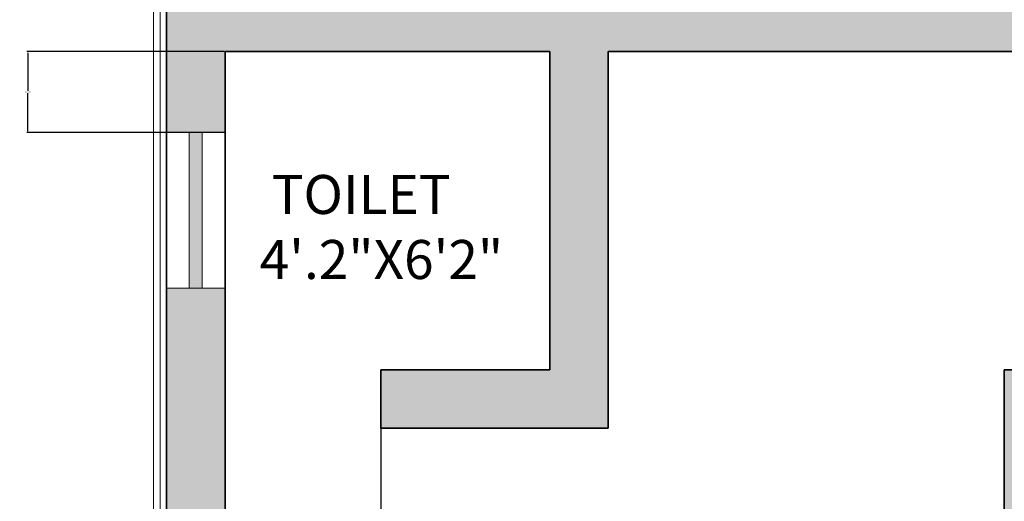
# Model space of a CAD drawing. Units: inches. Extents: x 311 to 815, y -527 to 136.
# Tile 6 of 21: x 388 to 539, y -368 to -294. Entities that reach past the tile are written whole.
import ezdxf

# ---------------------------------------------------------------- set-up
doc = ezdxf.new("R2010")
doc.units = ezdxf.units.IN
doc.header["$MEASUREMENT"] = 0
for name, color, linetype, lineweight in [('A-ANNO-DIMS', 1, 'Continuous', 18), ('A-AREA-IDEN', 8, 'Continuous', 18), ('A-FLOR-EDGE', 1, 'Continuous', 18), ('A-GLAZ-PATT', 5, 'Continuous', 13), ('A-WALL-PATT', 242, 'Continuous', 13), ('wall', 1, 'Continuous', 35), ('win', 5, 'Continuous', 18)]:
    doc.layers.add(name, color=color, linetype=linetype, lineweight=lineweight)
doc.styles.get("Standard").update_dxf_attribs({"font": 'arial.ttf'})
doc.dimstyles.get("Standard").update_dxf_attribs({"dimtxt": 0.18, "dimasz": 0.18, "dimexe": 0.18, "dimexo": 0.0625, "dimgap": 0.09, "dimtad": 0, "dimtih": 1, "dimtoh": 1, "dimdec": 1, "dimzin": 0, "dimdsep": 46, "dimlunit": 4, "dimtxsty": 'Standard', "dimcen": 0.09, "dimadec": 0, "dimazin": 0, "dimtfac": 1, "dimtdec": 1, "dimtofl": 0, "dimtmove": 0, "dimatfit": 3, "dimfxl": 1, "dimtolj": 1, "dimtzin": 0, "dimarcsym": 0})

# ---------------------------------------------------------------- blocks, each defined once
blk = doc.blocks.new('_ArchTick')
at = {"color": 0, "linetype": 'ByBlock', "const_width": 0.15}
blk.add_lwpolyline([(-0.5, -0.5), (0.5, 0.5)], dxfattribs=at)
blk = doc.blocks.new('_Oblique')
at = {"color": 0, "linetype": 'ByBlock', "lineweight": -2}
blk.add_line((-0.5, -0.5), (0.5, 0.5), dxfattribs=at)
blk = doc.blocks.new('*D3')
at = {"layer": 'A-ANNO-DIMS', "color": 0, "lineweight": -2, "transparency": 16777216}
for p, q in [((377.54, 21.87), (377.54, -221.61)), ((377.54, -482.13), (377.54, -238.65))]:
    blk.add_line(p, q, dxfattribs=at)
at = {"layer": 'Defpoints', "color": 0, "transparency": 16777216}
for p in [(410.32, 21.87), (377.54, -482.13), (410.32, -482.13)]:
    blk.add_point(p, dxfattribs=at)
at = {"layer": 'A-ANNO-DIMS', "color": 0, "lineweight": -2, "transparency": 16777216, "xscale": 9, "yscale": 9, "zscale": 9}
for name, p, rotation in [('_ArchTick', (377.54, 21.87), 90), ('_Oblique', (377.54, -482.13), 270)]:
    blk.add_blockref(name, p, dxfattribs=dict(at, rotation=rotation))
at = {"layer": 'A-ANNO-DIMS', "color": 0, "transparency": 16777216, "insert": (377.54, -230.13), "char_height": 9, "attachment_point": 5}
blk.add_mtext("\\A1;42'", dxfattribs=at)
blk = doc.blocks.new('WIN-24IN')
for p, q in [((9, 24), (0, 24)), ((3.5, 0), (3.5, 24)), ((5.5, 0), (5.5, 24)), ((9, 0), (0, 0))]:
    blk.add_line(p, q)
blk = doc.blocks.new('*D43')
at = {"layer": 'A-ANNO-DIMS', "color": 0, "lineweight": -2, "transparency": 16777216}
for p, q in [((419.26, -299.13), (388.79, -299.13)), ((388.97, -299.31), (388.97, -305.16)), ((388.97, -311.39), (388.97, -305.53)), ((419.26, -311.57), (388.79, -311.57))]:
    blk.add_line(p, q, dxfattribs=at)
at = {"layer": 'A-ANNO-DIMS', "color": 0, "transparency": 16777216}
for points in [[(388.94, -299.31), (389, -299.31), (388.97, -299.13)], [(388.94, -311.39), (389, -311.39), (388.97, -311.57)]]:
    blk.add_solid(points, dxfattribs=at)
at = {"layer": 'Defpoints', "color": 0, "transparency": 16777216}
for p in [(388.97, -299.13), (419.32, -299.13), (419.32, -311.57)]:
    blk.add_point(p, dxfattribs=at)
at = {"layer": 'A-ANNO-DIMS', "color": 0, "transparency": 16777216, "insert": (388.97, -305.35), "char_height": 0.18, "attachment_point": 5}
blk.add_mtext('\\A1;1\'-0 1/2"', dxfattribs=at)
blk = doc.blocks.new('*D54')
at = {"layer": 'A-ANNO-DIMS', "color": 0, "lineweight": -2, "transparency": 16777216}
for p, q in [((419.32, -335.63), (419.32, -526.66)), ((443.32, -348.19), (443.32, -526.66)), ((419.5, -526.48), (430.99, -526.48)), ((443.14, -526.48), (431.65, -526.48))]:
    blk.add_line(p, q, dxfattribs=at)
at = {"layer": 'A-ANNO-DIMS', "color": 0, "transparency": 16777216}
for points in [[(419.5, -526.45), (419.5, -526.51), (419.32, -526.48)], [(443.14, -526.45), (443.14, -526.51), (443.32, -526.48)]]:
    blk.add_solid(points, dxfattribs=at)
at = {"layer": 'Defpoints', "color": 0, "transparency": 16777216}
for p in [(419.32, -335.57), (443.32, -348.13), (443.32, -526.48)]:
    blk.add_point(p, dxfattribs=at)
at = {"layer": 'A-ANNO-DIMS', "color": 0, "transparency": 16777216, "insert": (431.32, -526.48), "char_height": 0.18, "attachment_point": 5}
blk.add_mtext('\\A1;2\'-0"', dxfattribs=at)

msp = doc.modelspace()

# ---------------------------------------------------------------- hatches: boundary and pattern name
at = {"layer": 'A-GLAZ-PATT'}
h = msp.add_hatch(color=256, dxfattribs=at)
h.dxf.hatch_style = 1
h.paths.add_polyline_path([(415.82, -202.13), (413.82, -202.13), (413.82, -262.13), (415.82, -262.13)])
h.paths.add_polyline_path([(415.82, -390.84), (413.82, -390.84), (413.82, -450.84), (415.82, -450.84)])
h.paths.add_polyline_path([(415.82, -311.57), (413.82, -311.57), (413.82, -335.57), (415.82, -335.57)])
h.paths.add_polyline_path([(509.32, -476.63), (449.32, -476.63), (449.32, -478.63), (509.32, -478.63)])
h.paths.add_polyline_path([(606.82, -476.63), (582.82, -476.63), (582.82, -478.63), (606.82, -478.63)])
h.paths.add_polyline_path([(678.82, -476.63), (654.82, -476.63), (654.82, -478.63), (678.82, -478.63)])
h.paths.add_polyline_path([(718.82, -385.13), (716.82, -385.13), (716.82, -445.13), (718.82, -445.13)])
h.paths.add_polyline_path([(718.82, -262.63), (716.82, -262.63), (716.82, -322.63), (718.82, -322.63)])
h.paths.add_polyline_path([(718.82, -140.13), (716.82, -140.13), (716.82, -200.13), (718.82, -200.13)])
h.paths.add_polyline_path([(718.82, -18.13), (716.82, -18.13), (716.82, -42.13), (718.82, -42.13)])
h.paths.add_polyline_path([(686.82, 18.37), (626.82, 18.37), (626.82, 16.37), (686.82, 16.37)])
h.paths.add_polyline_path([(581.82, 18.37), (557.82, 18.37), (557.82, 16.37), (581.82, 16.37)])
h.paths.add_polyline_path([(509.32, 18.37), (449.32, 18.37), (449.32, 16.37), (509.32, 16.37)])
at = {"layer": 'A-WALL-PATT'}
h = msp.add_hatch(color=256, dxfattribs=at)
h.dxf.hatch_style = 1
h.paths.add_polyline_path([(557.82, 21.87), (509.32, 21.87), (509.32, 12.87), (539.32, 12.87), (539.32, -112.13), (548.32, -112.13), (548.32, -58.63), (557.82, -58.63), (557.82, -49.63), (548.32, -49.63), (548.32, 12.87), (557.82, 12.87)])
h.paths.add_polyline_path([(449.32, 21.87), (410.32, 21.87), (410.32, -15.13), (419.32, -15.13), (419.32, 12.87), (449.32, 12.87)])
h.paths.add_polyline_path([(626.82, 21.87), (581.82, 21.87), (581.82, 12.87), (591.32, 12.87), (591.32, -49.63), (581.82, -49.63), (581.82, -58.63), (591.32, -58.63), (591.32, -112.13), (600.32, -112.13), (600.32, 12.87), (626.82, 12.87)])
h.paths.add_polyline_path([(722.32, 21.87), (686.82, 21.87), (686.82, 12.87), (713.32, 12.87), (713.32, -18.13), (722.32, -18.13)])
h.paths.add_polyline_path([(722.32, -42.13), (713.32, -42.13), (713.32, -73.13), (722.32, -73.13)])
h.paths.add_polyline_path([(501.32, -103.13), (419.32, -103.13), (419.32, -75.13), (410.32, -75.13), (410.32, -126.63), (419.32, -126.63), (419.32, -112.13), (492.32, -112.13), (492.32, -143.13), (501.32, -143.13)])
h.paths.add_polyline_path([(548.32, -165.13), (419.32, -165.13), (419.32, -150.63), (410.32, -150.63), (410.32, -202.13), (419.32, -202.13), (419.32, -174.13), (548.32, -174.13)])
h.paths.add_polyline_path([(722.32, -103.13), (636.32, -103.13), (636.32, -112.13), (713.32, -112.13), (713.32, -140.13), (722.32, -140.13)])
h.paths.add_polyline_path([(548.32, -210.13), (539.32, -210.13), (539.32, -290.13), (419.32, -290.13), (419.32, -262.13), (410.32, -262.13), (410.32, -311.57), (419.32, -311.57), (419.32, -299.13), (469.32, -299.13), (469.32, -348.13), (443.32, -348.13), (443.32, -357.13), (478.32, -357.13), (478.32, -299.13), (548.32, -299.13)])
h.paths.add_polyline_path([(722.32, -200.13), (713.32, -200.13), (713.32, -228.13), (609.32, -228.13), (609.32, -237.13), (713.32, -237.13), (713.32, -262.63), (722.32, -262.63)])
h.paths.add_polyline_path([(722.32, -322.63), (713.32, -322.63), (713.32, -348.13), (633.32, -348.13), (633.32, -357.13), (713.32, -357.13), (713.32, -385.13), (722.32, -385.13)])
h.paths.add_polyline_path([(419.32, -335.57), (410.32, -335.57), (410.32, -390.84), (419.32, -390.84)])
h.paths.add_polyline_path([(419.32, -450.84), (410.32, -450.84), (410.32, -482.13), (449.32, -482.13), (449.32, -473.13), (419.32, -473.13)])
h.paths.add_polyline_path([(582.82, -473.13), (548.32, -473.13), (548.32, -348.13), (539.32, -348.13), (539.32, -473.13), (509.32, -473.13), (509.32, -482.13), (582.82, -482.13)])
h.paths.add_polyline_path([(722.32, -445.13), (713.32, -445.13), (713.32, -473.13), (678.82, -473.13), (678.82, -482.13), (722.32, -482.13)])

# ---------------------------------------------------------------- linework, layer by layer
at = {"layer": 'A-FLOR-EDGE'}
for p, q in [((408.32, -484.13), (408.32, 23.87)), ((409.32, -483.13), (409.32, 22.87))]:
    msp.add_line(p, q, dxfattribs=at)
at = {"layer": 'wall'}
for p, q in [((410.32, -482.13), (410.32, 21.87)), ((419.32, -473.13), (419.32, -299.13)), ((469.32, -299.13), (419.32, -299.13)), ((469.32, -348.13), (469.32, -299.13)), ((548.32, -299.13), (478.32, -299.13)), ((478.32, -357.13), (478.32, -299.13)), ((443.32, -348.13), (469.32, -348.13)), ((443.32, -348.13), (469.32, -348.13)), ((443.32, -357.13), (443.32, -348.13)), ((539.32, -473.13), (539.32, -348.13)), ((539.32, -348.13), (548.32, -348.13)), ((539.32, -348.13), (548.32, -348.13)), ((443.32, -357.13), (478.32, -357.13)), ((443.32, -357.13), (478.32, -357.13))]:
    msp.add_line(p, q, dxfattribs=at)

# ---------------------------------------------------------------- block references
at = {"layer": 'win'}
msp.add_blockref('WIN-24IN', (410.32, -335.57), dxfattribs=at)

# ---------------------------------------------------------------- texts
at = {"layer": 'A-AREA-IDEN', "insert": (419.15, -318.13), "char_height": 6.0073, "attachment_point": 1}
msp.add_mtext_dynamic_manual_height_columns('    TOILET\\P   4\'.2"X6\'2"', width=54.4429, gutter_width=1, heights=[0], dxfattribs=at)

# ---------------------------------------------------------------- dimensions: what is measured, and where the dimension line sits
at = {"layer": 'A-ANNO-DIMS'}
for base, p1, p2, override, picture, middle in [((377.54, -482.13), (410.32, 21.87), (410.32, -482.13), {"dimtxt": 9, "dimasz": 9, "dimgap": 4, "dimblk1": 'ArchTick', "dimblk2": 'Oblique', "dimsah": 1, "dimse1": 1, "dimse2": 1, "dimclrd": 0, "dimclre": 0, "dimclrt": 0}, '*D3', (377.54, -230.13)), ((388.97, -299.13), (419.32, -311.57), (419.32, -299.13), {"dimdec": 1, "dimlfac": 1, "dimrnd": 0, "dimzin": 1, "dimdsep": 46, "dimlunit": 4, "dimfrac": 2}, '*D43', (388.97, -305.35))]:
    dim = msp.add_linear_dim(base=base, p1=p1, p2=p2, angle=90, dimstyle='Standard', override=override, dxfattribs=at)
    dim.commit()
    dim.dimension.update_dxf_attribs({"geometry": picture, "text_midpoint": middle})
dim = msp.add_linear_dim(base=(443.32, -526.48), p1=(419.32, -335.57), p2=(443.32, -348.13), dimstyle='Standard', override={"dimdec": 1, "dimlfac": 1, "dimrnd": 0, "dimzin": 1, "dimdsep": 46, "dimlunit": 4, "dimfrac": 2}, dxfattribs=at)
dim.commit()
dim.dimension.update_dxf_attribs({"geometry": '*D54', "text_midpoint": (431.32, -526.48)})

doc.saveas('drawing.dxf')
